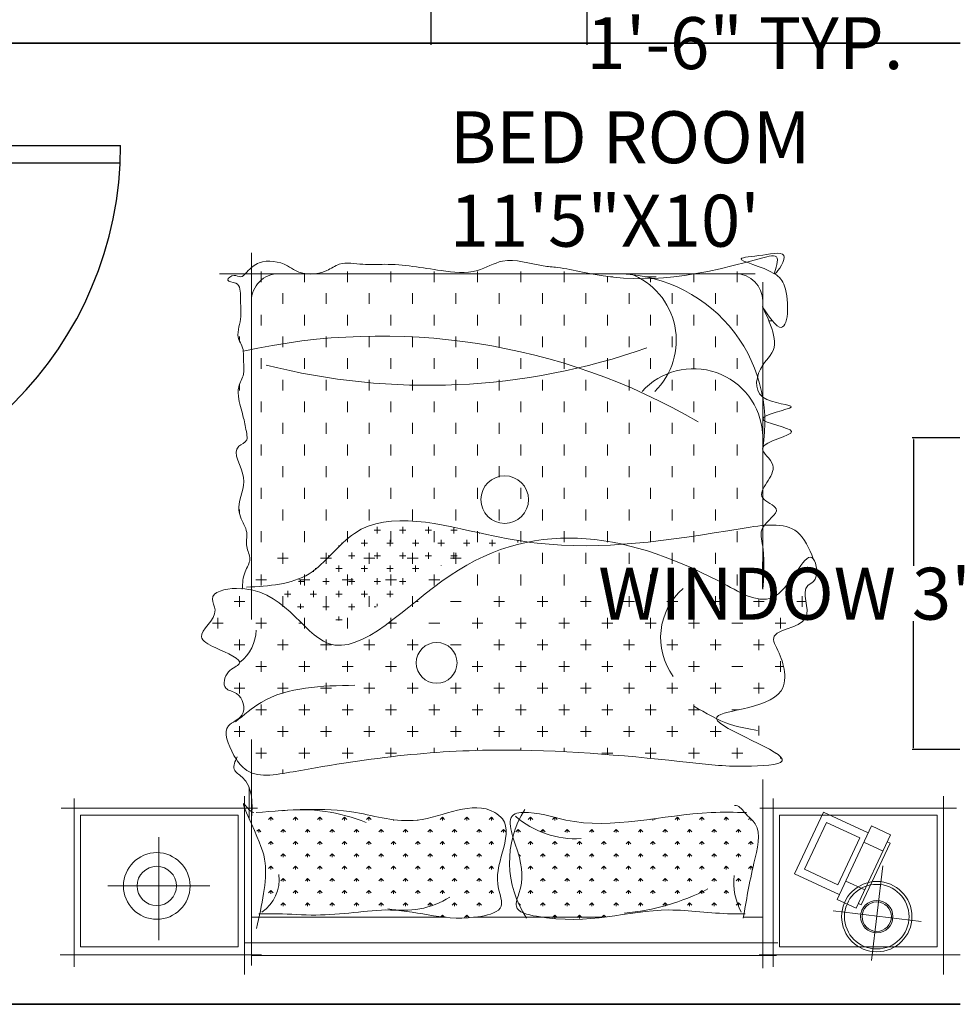
# Model space of a CAD drawing. Units: inches. Extents: x -26 to 575, y -18 to 513.
# Tile 17 of 28: x 405 to 513, y 128 to 241. Entities that reach past the tile are written whole.
import ezdxf

# ---------------------------------------------------------------- set-up
doc = ezdxf.new("R2010")
doc.units = ezdxf.units.IN
doc.header["$MEASUREMENT"] = 0
for name, color, linetype, lineweight in [('A-ANNO-DIMS', 2, 'Continuous', 18), ('A-AREA-IDEN', 7, 'Continuous', 18), ('A-DOOR', 3, 'Continuous', 25), ('A-WALL', 7, 'Continuous', 35), ('Furniture', 8, 'Continuous', 15)]:
    doc.layers.add(name, color=color, linetype=linetype, lineweight=lineweight)
doc.styles.get("Standard").update_dxf_attribs({"font": 'arial.ttf', "height": 6})
doc.dimstyles.get("Standard").update_dxf_attribs({"dimtxt": 6, "dimasz": 0.18, "dimexe": 0.18, "dimexo": 0.0625, "dimgap": 0.09, "dimtad": 0, "dimtih": 1, "dimtoh": 1, "dimzin": 0, "dimdsep": 46, "dimlunit": 3, "dimtxsty": 'Standard', "dimcen": 0.09, "dimadec": 0, "dimazin": 0, "dimtfac": 1, "dimtofl": 0, "dimtmove": 0, "dimatfit": 3, "dimfxl": 1, "dimtolj": 1, "dimtzin": 0, "dimarcsym": 0})

# ---------------------------------------------------------------- blocks, each defined once
blk = doc.blocks.new('BED-DOUBLE-WITH-NIGHTSTANDS')
for p, q in [((1.93, 83.36), (1.93, 62.76)), ((82.67, 83.36), (82.67, 62.76)), ((21.61, 63.03), (21.61, 82.46)), ((22.83, 60.83), (22.83, 82.62)), ((81.88, 82.34), (81.88, 56.23)), ((102.35, 63.03), (102.35, 82.46)), ((23.23, 81.08), (0, 81.08)), ((10.27, 81.76), (8.94, 70.83)), ((21.24, 81.17), (81.88, 81.17)), ((103.97, 81.08), (80.74, 81.08)), ((20.89, 80.15), (2.67, 80.15)), ((2.67, 80.15), (2.67, 64.97)), ((20.89, 64.97), (20.89, 80.15)), ((82.67, 79.72), (21.06, 79.72)), ((101.63, 80.15), (83.41, 80.15)), ((83.41, 80.15), (83.41, 64.97)), ((101.63, 64.97), (101.63, 80.15)), ((92.57, 79.4), (92.57, 67.51)), ((14.67, 76.01), (4.51, 77.26)), ((25.06, 76.76), (22.83, 76.76)), ((41.17, 76.51), (40.96, 76.72)), ((41.17, 76.51), (41.43, 76.77)), ((41.17, 76.51), (41.17, 76.74)), ((56.23, 76.76), (41.36, 76.76)), ((44, 76.51), (43.73, 76.77)), ((44, 76.51), (44, 76.88)), ((44, 76.51), (44.26, 76.77)), ((46.83, 76.51), (46.56, 76.77)), ((46.83, 76.51), (46.83, 76.88)), ((46.83, 76.51), (47.09, 76.77)), ((57, 76.51), (56.74, 76.77)), ((57, 76.51), (57, 76.83)), ((57, 76.51), (57.27, 76.77)), ((81.88, 76.76), (59.39, 76.76)), ((59.83, 76.51), (59.59, 76.74)), ((59.83, 76.51), (59.83, 76.72)), ((59.83, 76.51), (60.02, 76.69)), ((8.06, 67.24), (12.03, 75.72)), ((11.46, 75.32), (8.12, 68.2)), ((11.77, 75.18), (11.46, 75.32)), ((12.03, 75.72), (14.23, 74.69)), ((25.61, 75.09), (25.35, 75.36)), ((25.61, 75.09), (25.61, 75.47)), ((25.61, 75.09), (25.88, 75.36)), ((28.44, 75.09), (28.18, 75.36)), ((28.44, 75.09), (28.44, 75.47)), ((28.44, 75.09), (28.71, 75.36)), ((31.27, 75.09), (31, 75.36)), ((31.27, 75.09), (31.27, 75.47)), ((31.27, 75.09), (31.53, 75.36)), ((34.1, 75.09), (33.83, 75.36)), ((34.1, 75.09), (34.1, 75.47)), ((34.1, 75.09), (34.36, 75.36)), ((36.93, 75.09), (36.66, 75.36)), ((36.93, 75.09), (36.93, 75.47)), ((36.93, 75.09), (37.19, 75.36)), ((39.75, 75.09), (39.49, 75.36)), ((39.75, 75.09), (39.75, 75.47)), ((39.75, 75.09), (40.02, 75.36)), ((42.58, 75.09), (42.32, 75.36)), ((42.58, 75.09), (42.58, 75.47)), ((42.58, 75.09), (42.85, 75.36)), ((45.41, 75.09), (45.15, 75.36)), ((45.41, 75.09), (45.41, 75.47)), ((45.41, 75.09), (45.68, 75.36)), ((48.24, 75.09), (47.97, 75.36)), ((48.24, 75.09), (48.24, 75.47)), ((48.24, 75.09), (48.5, 75.36)), ((51.07, 75.09), (50.8, 75.36)), ((51.07, 75.09), (51.07, 75.1)), ((51.07, 75.09), (51.07, 75.1)), ((53, 75.34), (53.03, 75.36)), ((55.59, 75.09), (55.32, 75.36)), ((55.59, 75.09), (55.59, 75.47)), ((55.59, 75.09), (55.85, 75.36)), ((58.42, 75.09), (58.15, 75.36)), ((58.42, 75.09), (58.42, 75.47)), ((58.42, 75.09), (58.68, 75.36)), ((61.25, 75.09), (60.98, 75.36)), ((61.25, 75.09), (61.25, 75.47)), ((61.25, 75.09), (61.51, 75.36)), ((64.07, 75.09), (63.81, 75.36)), ((64.07, 75.09), (64.07, 75.47)), ((64.07, 75.09), (64.34, 75.36)), ((66.9, 75.09), (66.64, 75.36)), ((66.9, 75.09), (66.9, 75.47)), ((66.9, 75.09), (67.17, 75.36)), ((69.73, 75.09), (69.47, 75.36)), ((69.73, 75.09), (69.73, 75.47)), ((69.73, 75.09), (70, 75.36)), ((72.56, 75.09), (72.29, 75.36)), ((72.56, 75.09), (72.56, 75.47)), ((72.56, 75.09), (72.82, 75.36)), ((75.39, 75.09), (75.12, 75.36)), ((75.39, 75.09), (75.39, 75.47)), ((75.39, 75.09), (75.65, 75.36)), ((78.22, 75.09), (77.95, 75.36)), ((78.22, 75.09), (78.22, 75.47)), ((78.22, 75.09), (78.48, 75.36)), ((14.23, 74.69), (10.26, 66.21)), ((19.14, 71.73), (13.98, 74.14)), ((27.03, 73.68), (26.76, 73.94)), ((27.03, 73.68), (27.03, 74.05)), ((27.03, 73.68), (27.29, 73.94)), ((29.85, 73.68), (29.59, 73.94)), ((29.85, 73.68), (30.12, 73.94)), ((29.86, 73.68), (29.86, 74.05)), ((32.68, 73.68), (32.42, 73.94)), ((32.68, 73.68), (32.68, 74.05)), ((32.68, 73.68), (32.95, 73.94)), ((35.51, 73.68), (35.25, 73.94)), ((35.51, 73.68), (35.51, 74.05)), ((35.51, 73.68), (35.78, 73.94)), ((38.34, 73.68), (38.07, 73.94)), ((38.34, 73.68), (38.34, 74.05)), ((38.34, 73.68), (38.61, 73.94)), ((41.17, 73.68), (40.9, 73.94)), ((41.17, 73.68), (41.17, 74.05)), ((41.17, 73.68), (41.43, 73.94)), ((44, 73.68), (43.73, 73.94)), ((44, 73.68), (44, 74.05)), ((44, 73.68), (44.26, 73.94)), ((46.83, 73.68), (46.56, 73.94)), ((46.83, 73.68), (46.83, 74.05)), ((46.83, 73.68), (47.09, 73.94)), ((49.65, 73.68), (49.39, 73.94)), ((49.65, 73.68), (49.65, 74.05)), ((49.65, 73.68), (49.92, 73.94)), ((54.17, 73.68), (53.91, 73.94)), ((54.17, 73.68), (54.17, 74.05)), ((54.17, 73.68), (54.44, 73.94)), ((57, 73.68), (56.74, 73.94)), ((57, 73.68), (57, 74.05)), ((57, 73.68), (57.27, 73.94)), ((59.83, 73.68), (59.57, 73.94)), ((59.83, 73.68), (59.83, 74.05)), ((59.83, 73.68), (60.1, 73.94)), ((62.66, 73.68), (62.39, 73.94)), ((62.66, 73.68), (62.66, 74.05)), ((62.66, 73.68), (62.92, 73.94)), ((65.49, 73.68), (65.22, 73.94)), ((65.49, 73.68), (65.49, 74.05)), ((65.49, 73.68), (65.75, 73.94)), ((68.32, 73.68), (68.05, 73.94)), ((68.32, 73.68), (68.32, 74.05)), ((68.32, 73.68), (68.58, 73.94)), ((71.14, 73.68), (70.88, 73.94)), ((71.14, 73.68), (71.41, 73.94)), ((71.15, 73.68), (71.15, 74.05)), ((73.97, 73.68), (73.71, 73.94)), ((73.97, 73.68), (73.97, 74.05)), ((73.97, 73.68), (74.24, 73.94)), ((76.8, 73.68), (76.54, 73.94)), ((76.8, 73.68), (76.8, 74.05)), ((76.8, 73.68), (77.07, 73.94)), ((79.63, 73.68), (79.36, 73.94)), ((79.63, 73.68), (79.63, 74.05)), ((79.63, 73.68), (79.9, 73.94)), ((13.24, 72.57), (11.03, 73.6)), ((14.13, 73), (11.6, 67.59)), ((17.98, 71.2), (14.13, 73)), ((98.47, 73.14), (86.67, 73.14)), ((15.8, 64.6), (19.14, 71.73)), ((25.61, 72.26), (25.35, 72.53)), ((25.61, 72.26), (25.61, 72.64)), ((25.61, 72.26), (25.88, 72.53)), ((28.44, 72.26), (28.18, 72.53)), ((28.44, 72.26), (28.44, 72.64)), ((28.44, 72.26), (28.71, 72.53)), ((31.27, 72.26), (31, 72.53)), ((31.27, 72.26), (31.27, 72.64)), ((31.27, 72.26), (31.53, 72.53)), ((34.1, 72.26), (33.83, 72.53)), ((34.1, 72.26), (34.1, 72.64)), ((34.1, 72.26), (34.36, 72.53)), ((36.93, 72.26), (36.66, 72.53)), ((36.93, 72.26), (36.93, 72.64)), ((36.93, 72.26), (37.19, 72.53)), ((39.75, 72.26), (39.49, 72.53)), ((39.75, 72.26), (39.75, 72.64)), ((39.75, 72.26), (40.02, 72.53)), ((42.58, 72.26), (42.32, 72.53)), ((42.58, 72.26), (42.58, 72.64)), ((42.58, 72.26), (42.85, 72.53)), ((45.41, 72.26), (45.15, 72.53)), ((45.41, 72.26), (45.41, 72.64)), ((45.41, 72.26), (45.68, 72.53)), ((48.24, 72.26), (47.97, 72.53)), ((48.24, 72.26), (48.24, 72.64)), ((48.24, 72.26), (48.5, 72.53)), ((55.59, 72.26), (55.32, 72.53)), ((55.59, 72.26), (55.59, 72.64)), ((55.59, 72.26), (55.85, 72.53)), ((58.42, 72.26), (58.15, 72.53)), ((58.42, 72.26), (58.42, 72.64)), ((58.42, 72.26), (58.68, 72.53)), ((61.25, 72.26), (60.98, 72.53)), ((61.25, 72.26), (61.25, 72.64)), ((61.25, 72.26), (61.51, 72.53)), ((64.07, 72.26), (63.81, 72.53)), ((64.07, 72.26), (64.07, 72.64)), ((64.07, 72.26), (64.34, 72.53)), ((66.9, 72.26), (66.64, 72.53)), ((66.9, 72.26), (66.9, 72.64)), ((66.9, 72.26), (67.17, 72.53)), ((69.73, 72.26), (69.47, 72.53)), ((69.73, 72.26), (69.73, 72.64)), ((69.73, 72.26), (70, 72.53)), ((72.56, 72.26), (72.29, 72.53)), ((72.56, 72.26), (72.56, 72.64)), ((72.56, 72.26), (72.82, 72.53)), ((75.39, 72.26), (75.12, 72.53)), ((75.39, 72.26), (75.39, 72.64)), ((75.39, 72.26), (75.65, 72.53)), ((78.22, 72.26), (77.95, 72.53)), ((78.22, 72.26), (78.22, 72.64)), ((78.22, 72.26), (78.48, 72.53)), ((15.45, 65.79), (17.98, 71.2)), ((24.2, 70.85), (23.97, 71.08)), ((24.2, 70.85), (24.2, 71.23)), ((24.2, 70.85), (24.46, 71.12)), ((27.03, 70.85), (26.76, 71.12)), ((27.03, 70.85), (27.03, 71.23)), ((27.03, 70.85), (27.29, 71.12)), ((29.85, 70.85), (29.59, 71.12)), ((29.85, 70.85), (30.12, 71.12)), ((29.86, 70.85), (29.86, 71.23)), ((32.68, 70.85), (32.42, 71.12)), ((32.68, 70.85), (32.68, 71.23)), ((32.68, 70.85), (32.95, 71.12)), ((35.51, 70.85), (35.25, 71.12)), ((35.51, 70.85), (35.51, 71.23)), ((35.51, 70.85), (35.78, 71.12)), ((38.34, 70.85), (38.07, 71.12)), ((38.34, 70.85), (38.34, 71.23)), ((38.34, 70.85), (38.61, 71.12)), ((41.17, 70.85), (40.9, 71.12)), ((41.17, 70.85), (41.17, 71.23)), ((41.17, 70.85), (41.43, 71.12)), ((44, 70.85), (43.73, 71.12)), ((44, 70.85), (44, 71.23)), ((44, 70.85), (44.26, 71.12)), ((46.83, 70.85), (46.56, 71.12)), ((46.83, 70.85), (46.83, 71.23)), ((46.83, 70.85), (47.09, 71.12)), ((49.65, 70.85), (49.39, 71.12)), ((49.65, 70.85), (49.65, 71.23)), ((49.65, 70.85), (49.92, 71.12)), ((54.17, 70.85), (53.91, 71.12)), ((54.17, 70.85), (54.17, 71.23)), ((54.17, 70.85), (54.44, 71.12)), ((57, 70.85), (56.74, 71.12)), ((57, 70.85), (57, 71.23)), ((57, 70.85), (57.27, 71.12)), ((59.83, 70.85), (59.57, 71.12)), ((59.83, 70.85), (59.83, 71.23)), ((59.83, 70.85), (60.1, 71.12)), ((62.66, 70.85), (62.39, 71.12)), ((62.66, 70.85), (62.66, 71.23)), ((62.66, 70.85), (62.92, 71.12)), ((65.49, 70.85), (65.22, 71.12)), ((65.49, 70.85), (65.49, 71.23)), ((65.49, 70.85), (65.75, 71.12)), ((68.32, 70.85), (68.05, 71.12)), ((68.32, 70.85), (68.32, 71.23)), ((68.32, 70.85), (68.58, 71.12)), ((71.14, 70.85), (70.88, 71.12)), ((71.14, 70.85), (71.41, 71.12)), ((71.15, 70.85), (71.15, 71.23)), ((73.97, 70.85), (73.71, 71.12)), ((73.97, 70.85), (73.97, 71.23)), ((73.97, 70.85), (74.24, 71.12)), ((76.8, 70.85), (76.54, 71.12)), ((76.8, 70.85), (76.8, 71.23)), ((76.8, 70.85), (77.07, 71.12)), ((79.63, 70.85), (79.36, 71.12)), ((79.63, 70.85), (79.63, 71.23)), ((79.63, 70.85), (79.9, 71.12)), ((25.61, 69.44), (25.35, 69.7)), ((25.61, 69.44), (25.61, 69.81)), ((25.61, 69.44), (25.88, 69.7)), ((28.44, 69.44), (28.18, 69.7)), ((28.44, 69.44), (28.44, 69.81)), ((28.44, 69.44), (28.71, 69.7)), ((31.27, 69.44), (31, 69.7)), ((31.27, 69.44), (31.27, 69.81)), ((31.27, 69.44), (31.53, 69.7)), ((34.1, 69.44), (33.83, 69.7)), ((34.1, 69.44), (34.1, 69.81)), ((34.1, 69.44), (34.36, 69.7)), ((36.93, 69.44), (36.66, 69.7)), ((36.93, 69.44), (36.93, 69.81)), ((36.93, 69.44), (37.19, 69.7)), ((39.75, 69.44), (39.49, 69.7)), ((39.75, 69.44), (39.75, 69.81)), ((39.75, 69.44), (40.02, 69.7)), ((42.58, 69.44), (42.32, 69.7)), ((42.58, 69.44), (42.58, 69.81)), ((42.58, 69.44), (42.85, 69.7)), ((45.41, 69.44), (45.15, 69.7)), ((45.41, 69.44), (45.41, 69.81)), ((45.41, 69.44), (45.68, 69.7)), ((48.24, 69.44), (47.97, 69.7)), ((48.24, 69.44), (48.24, 69.81)), ((48.24, 69.44), (48.5, 69.7)), ((51.05, 69.45), (50.8, 69.7)), ((53.01, 69.68), (53.03, 69.7)), ((55.59, 69.44), (55.32, 69.7)), ((55.59, 69.44), (55.59, 69.81)), ((55.59, 69.44), (55.85, 69.7)), ((58.42, 69.44), (58.15, 69.7)), ((58.42, 69.44), (58.42, 69.81)), ((58.42, 69.44), (58.68, 69.7)), ((61.25, 69.44), (60.98, 69.7)), ((61.25, 69.44), (61.25, 69.81)), ((61.25, 69.44), (61.51, 69.7)), ((64.07, 69.44), (63.81, 69.7)), ((64.07, 69.44), (64.07, 69.81)), ((64.07, 69.44), (64.34, 69.7)), ((66.9, 69.44), (66.64, 69.7)), ((66.9, 69.44), (66.9, 69.81)), ((66.9, 69.44), (67.17, 69.7)), ((69.73, 69.44), (69.47, 69.7)), ((69.73, 69.44), (69.73, 69.81)), ((69.73, 69.44), (70, 69.7)), ((72.56, 69.44), (72.29, 69.7)), ((72.56, 69.44), (72.56, 69.81)), ((72.56, 69.44), (72.82, 69.7)), ((75.39, 69.44), (75.12, 69.7)), ((75.39, 69.44), (75.39, 69.81)), ((75.39, 69.44), (75.65, 69.7)), ((78.22, 69.44), (77.95, 69.7)), ((78.22, 69.44), (78.22, 69.81)), ((78.22, 69.44), (78.48, 69.7)), ((11.14, 68.07), (8.93, 69.1)), ((24.2, 68.02), (23.93, 68.29)), ((24.2, 68.02), (24.2, 68.4)), ((24.2, 68.02), (24.46, 68.29)), ((27.03, 68.02), (26.76, 68.29)), ((27.03, 68.02), (27.03, 68.4)), ((27.03, 68.02), (27.29, 68.29)), ((29.85, 68.02), (29.59, 68.29)), ((29.85, 68.02), (30.12, 68.29)), ((29.86, 68.02), (29.86, 68.4)), ((32.68, 68.02), (32.42, 68.29)), ((32.68, 68.02), (32.68, 68.4)), ((32.68, 68.02), (32.95, 68.29)), ((35.51, 68.02), (35.25, 68.29)), ((35.51, 68.02), (35.51, 68.4)), ((35.51, 68.02), (35.78, 68.29)), ((38.34, 68.02), (38.07, 68.29)), ((38.34, 68.02), (38.34, 68.4)), ((38.34, 68.02), (38.61, 68.29)), ((41.17, 68.02), (40.9, 68.29)), ((41.17, 68.02), (41.17, 68.4)), ((41.17, 68.02), (41.43, 68.29)), ((44, 68.02), (43.73, 68.29)), ((44, 68.02), (44, 68.4)), ((44, 68.02), (44.26, 68.29)), ((46.83, 68.02), (46.56, 68.29)), ((46.83, 68.02), (46.83, 68.4)), ((46.83, 68.02), (47.09, 68.29)), ((49.65, 68.02), (49.39, 68.29)), ((49.65, 68.02), (49.65, 68.4)), ((49.65, 68.02), (49.92, 68.29)), ((54.17, 68.02), (53.91, 68.29)), ((54.17, 68.02), (54.17, 68.4)), ((54.17, 68.02), (54.44, 68.29)), ((57, 68.02), (56.74, 68.29)), ((57, 68.02), (57, 68.4)), ((57, 68.02), (57.27, 68.29)), ((59.83, 68.02), (59.57, 68.29)), ((59.83, 68.02), (59.83, 68.4)), ((59.83, 68.02), (60.1, 68.29)), ((62.66, 68.02), (62.39, 68.29)), ((62.66, 68.02), (62.66, 68.4)), ((62.66, 68.02), (62.92, 68.29)), ((65.49, 68.02), (65.22, 68.29)), ((65.49, 68.02), (65.49, 68.4)), ((65.49, 68.02), (65.75, 68.29)), ((68.32, 68.02), (68.05, 68.29)), ((68.32, 68.02), (68.32, 68.4)), ((68.32, 68.02), (68.58, 68.29)), ((71.14, 68.02), (70.88, 68.29)), ((71.14, 68.02), (71.41, 68.29)), ((71.15, 68.02), (71.15, 68.4)), ((73.97, 68.02), (73.71, 68.29)), ((73.97, 68.02), (73.97, 68.4)), ((73.97, 68.02), (74.24, 68.29)), ((76.8, 68.02), (76.54, 68.29)), ((76.8, 68.02), (76.8, 68.4)), ((76.8, 68.02), (77.07, 68.29)), ((79.63, 68.02), (79.36, 68.29)), ((79.63, 68.02), (79.63, 68.4)), ((79.63, 68.02), (79.9, 68.29)), ((10.26, 66.21), (8.06, 67.24)), ((8.12, 68.2), (8.43, 68.05)), ((11.6, 67.59), (15.45, 65.79)), ((10.64, 67.02), (15.8, 64.6)), ((25.61, 66.61), (25.35, 66.87)), ((25.61, 66.61), (25.61, 66.98)), ((25.61, 66.61), (25.88, 66.87)), ((28.44, 66.61), (28.18, 66.87)), ((28.44, 66.61), (28.44, 66.98)), ((28.44, 66.61), (28.71, 66.87)), ((31.27, 66.61), (31, 66.87)), ((31.27, 66.61), (31.27, 66.98)), ((31.27, 66.61), (31.53, 66.87)), ((34.1, 66.61), (33.83, 66.87)), ((34.1, 66.61), (34.1, 66.98)), ((34.1, 66.61), (34.36, 66.87)), ((36.93, 66.61), (36.66, 66.87)), ((36.93, 66.61), (36.93, 66.98)), ((36.93, 66.61), (37.19, 66.87)), ((39.75, 66.61), (39.49, 66.87)), ((39.75, 66.61), (39.75, 66.98)), ((39.75, 66.61), (40.02, 66.87)), ((42.58, 66.61), (42.32, 66.87)), ((42.58, 66.61), (42.58, 66.98)), ((42.58, 66.61), (42.85, 66.87)), ((45.41, 66.61), (45.15, 66.87)), ((45.41, 66.61), (45.41, 66.98)), ((45.41, 66.61), (45.68, 66.87)), ((48.24, 66.61), (47.97, 66.87)), ((48.24, 66.61), (48.24, 66.98)), ((48.24, 66.61), (48.5, 66.87)), ((51.07, 66.61), (50.8, 66.87)), ((51.07, 66.61), (51.07, 66.98)), ((51.07, 66.61), (51.33, 66.87)), ((52.76, 66.61), (52.49, 66.87)), ((52.76, 66.61), (52.76, 66.98)), ((52.76, 66.61), (53.03, 66.87)), ((55.59, 66.61), (55.32, 66.87)), ((55.59, 66.61), (55.59, 66.98)), ((55.59, 66.61), (55.85, 66.87)), ((58.42, 66.61), (58.15, 66.87)), ((58.42, 66.61), (58.42, 66.98)), ((58.42, 66.61), (58.68, 66.87)), ((61.25, 66.61), (60.98, 66.87)), ((61.25, 66.61), (61.25, 66.98)), ((61.25, 66.61), (61.51, 66.87)), ((64.07, 66.61), (63.81, 66.87)), ((64.07, 66.61), (64.07, 66.98)), ((64.07, 66.61), (64.34, 66.87)), ((66.9, 66.61), (66.64, 66.87)), ((66.9, 66.61), (66.9, 66.98)), ((66.9, 66.61), (67.17, 66.87)), ((69.73, 66.61), (69.47, 66.87)), ((69.73, 66.61), (69.73, 66.98)), ((69.73, 66.61), (70, 66.87)), ((72.56, 66.61), (72.29, 66.87)), ((72.56, 66.61), (72.56, 66.98)), ((72.56, 66.61), (72.82, 66.87)), ((75.39, 66.61), (75.12, 66.87)), ((75.39, 66.61), (75.39, 66.98)), ((75.39, 66.61), (75.65, 66.87)), ((78.22, 66.61), (77.95, 66.87)), ((78.22, 66.61), (78.22, 66.98)), ((78.22, 66.61), (78.48, 66.87)), ((81.04, 66.61), (80.78, 66.87)), ((81.04, 66.61), (81.04, 66.98)), ((81.04, 66.61), (81.25, 66.82)), ((2.67, 64.97), (20.89, 64.97)), ((24.2, 65.39), (24.2, 65.57)), ((24.29, 65.29), (24.46, 65.46)), ((27.03, 65.19), (26.76, 65.46)), ((27.03, 65.19), (27.03, 65.57)), ((27.03, 65.19), (27.29, 65.46)), ((29.85, 65.19), (29.59, 65.46)), ((29.85, 65.19), (30.12, 65.46)), ((29.86, 65.19), (29.86, 65.57)), ((32.68, 65.19), (32.42, 65.46)), ((32.68, 65.19), (32.68, 65.57)), ((32.68, 65.19), (32.95, 65.46)), ((35.33, 65.37), (35.25, 65.46)), ((35.51, 65.39), (35.51, 65.57)), ((35.74, 65.42), (35.78, 65.46)), ((46.77, 65.25), (46.56, 65.46)), ((46.83, 65.23), (46.83, 65.57)), ((46.86, 65.22), (47.09, 65.46)), ((49.65, 65.19), (49.39, 65.46)), ((49.65, 65.19), (49.65, 65.57)), ((49.65, 65.19), (49.92, 65.46)), ((54.17, 65.19), (53.91, 65.46)), ((54.17, 65.19), (54.17, 65.57)), ((54.17, 65.19), (54.44, 65.46)), ((57, 65.19), (56.74, 65.46)), ((57, 65.19), (57, 65.57)), ((57, 65.19), (57.27, 65.46)), ((59.83, 65.19), (59.57, 65.46)), ((59.83, 65.19), (59.83, 65.57)), ((59.83, 65.19), (60.1, 65.46)), ((62.66, 65.52), (62.66, 65.57)), ((65.49, 65.48), (65.49, 65.57)), ((65.74, 65.45), (65.75, 65.46)), ((68.32, 65.19), (68.05, 65.46)), ((68.32, 65.19), (68.32, 65.57)), ((68.32, 65.19), (68.58, 65.46)), ((71.14, 65.19), (70.88, 65.46)), ((71.14, 65.19), (71.41, 65.46)), ((71.15, 65.19), (71.15, 65.57)), ((73.97, 65.19), (73.71, 65.46)), ((73.97, 65.19), (73.97, 65.57)), ((73.97, 65.19), (74.24, 65.46)), ((76.8, 65.19), (76.54, 65.46)), ((76.8, 65.19), (76.8, 65.57)), ((76.8, 65.19), (77.07, 65.46)), ((79.63, 65.19), (79.36, 65.46)), ((79.63, 65.19), (79.63, 65.57)), ((79.63, 65.19), (79.9, 65.46)), ((82.15, 61.74), (82.15, 65.42)), ((83.41, 64.97), (101.63, 64.97)), ((0.45, 64.15), (23.14, 64.15)), ((55.59, 64.12), (55.59, 64.15)), ((81.19, 64.15), (103.88, 64.15)), ((78.27, 59.67), (78.27, 60.15)), ((20.77, 58.21), (20.77, 58.42)), ((25.77, 57.17), (25.77, 58.42)), ((30.77, 57.17), (30.77, 58.42)), ((35.77, 57.17), (35.77, 58.41)), ((65.77, 57.17), (65.77, 58.21)), ((70.77, 57.17), (70.77, 58.42)), ((75.77, 57.17), (75.77, 58.42)), ((80.77, 57.17), (80.77, 58.42)), ((21.39, 57.79), (21.31, 57.79)), ((26.39, 57.79), (25.14, 57.79)), ((31.39, 57.79), (30.14, 57.79)), ((36.39, 57.79), (35.14, 57.79)), ((41.39, 57.79), (40.14, 57.79)), ((40.77, 57.17), (40.77, 57.97)), ((45.77, 57.17), (45.77, 57.64)), ((50.77, 57.17), (50.77, 57.46)), ((55.77, 57.17), (55.77, 57.48)), ((60.77, 57.17), (60.77, 57.74)), ((66.39, 57.79), (65.14, 57.79)), ((71.39, 57.79), (70.14, 57.79)), ((76.39, 57.79), (75.14, 57.79)), ((81.39, 57.79), (80.14, 57.79)), ((23.27, 54.64), (23.27, 55.76)), ((28.27, 54.67), (28.27, 55.92)), ((33.27, 54.67), (33.27, 55.92)), ((38.27, 54.67), (38.27, 55.92)), ((43.27, 54.67), (43.27, 55.92)), ((48.27, 54.67), (48.27, 55.92)), ((53.27, 54.67), (53.27, 55.92)), ((58.27, 54.67), (58.27, 55.92)), ((63.27, 54.67), (63.27, 55.92)), ((68.27, 54.67), (68.27, 55.92)), ((73.27, 54.67), (73.27, 55.92)), ((78.27, 54.67), (78.27, 55.92)), ((83.27, 54.67), (83.27, 55.92)), ((28.89, 55.29), (27.64, 55.29)), ((33.89, 55.29), (32.64, 55.29)), ((38.89, 55.29), (37.64, 55.29)), ((43.89, 55.29), (42.64, 55.29)), ((48.89, 55.29), (47.64, 55.29)), ((53.89, 55.29), (52.64, 55.29)), ((58.89, 55.29), (57.64, 55.29)), ((63.89, 55.29), (62.64, 55.29)), ((68.89, 55.29), (67.64, 55.29)), ((73.89, 55.29), (72.64, 55.29)), ((78.89, 55.29), (77.64, 55.29)), ((83.89, 55.29), (82.64, 55.29)), ((26.39, 52.79), (25.62, 52.79)), ((31.39, 52.79), (30.14, 52.79)), ((30.77, 52.17), (30.77, 53.42)), ((36.39, 52.79), (35.14, 52.79)), ((35.77, 52.17), (35.77, 53.42)), ((41.39, 52.79), (40.14, 52.79)), ((40.77, 52.17), (40.77, 53.42)), ((46.39, 52.79), (45.14, 52.79)), ((45.77, 52.17), (45.77, 53.42)), ((51.39, 52.79), (50.14, 52.79)), ((50.77, 52.17), (50.77, 53.42)), ((56.39, 52.79), (55.14, 52.79)), ((55.77, 52.17), (55.77, 53.42)), ((61.39, 52.79), (60.14, 52.79)), ((60.77, 52.17), (60.77, 53.42)), ((66.39, 52.79), (65.14, 52.79)), ((65.77, 52.17), (65.77, 53.42)), ((71.39, 52.79), (70.14, 52.79)), ((70.77, 52.17), (70.77, 53.42)), ((76.39, 52.79), (75.14, 52.79)), ((75.77, 52.17), (75.77, 53.42)), ((81.39, 52.79), (80.14, 52.79)), ((80.77, 52.17), (80.77, 53.42)), ((23.89, 50.29), (22.64, 50.29)), ((23.27, 49.67), (23.27, 50.92)), ((28.89, 50.29), (27.64, 50.29)), ((28.27, 49.67), (28.27, 50.92)), ((33.89, 50.29), (32.64, 50.29)), ((33.27, 49.67), (33.27, 50.92)), ((38.89, 50.29), (37.64, 50.29)), ((38.27, 49.67), (38.27, 50.92)), ((43.89, 50.29), (42.64, 50.29)), ((43.27, 49.67), (43.27, 50.92)), ((48.89, 50.29), (47.64, 50.29)), ((48.27, 49.67), (48.27, 50.92)), ((53.89, 50.29), (52.64, 50.29)), ((53.27, 49.67), (53.27, 50.92)), ((58.89, 50.29), (57.64, 50.29)), ((58.27, 49.67), (58.27, 50.92)), ((63.89, 50.29), (62.64, 50.29)), ((63.27, 49.67), (63.27, 50.92)), ((68.89, 50.29), (67.64, 50.29)), ((68.27, 49.67), (68.27, 50.92)), ((73.89, 50.29), (72.64, 50.29)), ((73.27, 49.67), (73.27, 50.92)), ((78.89, 50.29), (77.64, 50.29)), ((78.27, 49.67), (78.27, 50.92)), ((83.89, 50.29), (82.64, 50.29)), ((83.27, 49.67), (83.27, 50.92)), ((21.39, 47.79), (20.41, 47.79)), ((20.77, 47.17), (20.77, 48.42)), ((26.39, 47.79), (25.14, 47.79)), ((31.39, 47.79), (30.14, 47.79)), ((30.77, 47.17), (30.77, 48.42)), ((36.39, 47.79), (35.14, 47.79)), ((35.77, 47.17), (35.77, 48.42)), ((41.39, 47.79), (40.14, 47.79)), ((40.77, 47.17), (40.77, 48.42)), ((46.39, 47.79), (45.14, 47.79)), ((45.77, 47.17), (45.77, 48.42)), ((51.39, 47.79), (50.14, 47.79)), ((50.77, 47.17), (50.77, 48.42)), ((56.39, 47.79), (55.14, 47.79)), ((55.77, 47.17), (55.77, 48.42)), ((66.39, 47.79), (65.14, 47.79)), ((65.77, 47.17), (65.77, 48.42)), ((71.39, 47.79), (70.14, 47.79)), ((70.77, 47.17), (70.77, 48.42)), ((76.39, 47.79), (75.14, 47.79)), ((75.77, 47.17), (75.77, 48.42)), ((81.39, 47.79), (80.14, 47.79)), ((80.77, 47.17), (80.77, 48.42)), ((23.27, 44.67), (23.27, 45.92)), ((28.27, 44.67), (28.27, 45.92)), ((33.27, 44.67), (33.27, 45.92)), ((38.27, 44.67), (38.27, 45.92)), ((43.27, 44.67), (43.27, 45.92)), ((48.27, 44.67), (48.27, 45.92)), ((53.27, 44.67), (53.27, 45.92)), ((63.27, 44.67), (63.27, 45.92)), ((68.27, 44.67), (68.27, 45.92)), ((73.27, 44.67), (73.27, 45.92)), ((78.27, 44.67), (78.27, 45.92)), ((83.27, 44.67), (83.27, 45.92)), ((23.89, 45.29), (22.64, 45.29)), ((28.89, 45.29), (27.64, 45.29)), ((33.89, 45.29), (32.64, 45.29)), ((38.89, 45.29), (37.64, 45.29)), ((43.89, 45.29), (42.64, 45.29)), ((48.89, 45.29), (47.64, 45.29)), ((53.89, 45.29), (52.64, 45.29)), ((58.89, 45.29), (57.64, 45.29)), ((63.89, 45.29), (62.64, 45.29)), ((68.89, 45.29), (67.64, 45.29)), ((73.89, 45.29), (72.64, 45.29)), ((78.89, 45.29), (77.64, 45.29)), ((83.89, 45.29), (82.64, 45.29)), ((20.77, 42.17), (20.77, 43.42)), ((30.77, 42.17), (30.77, 43.42)), ((35.77, 42.17), (35.77, 43.42)), ((40.77, 42.17), (40.77, 43.42)), ((45.77, 42.17), (45.77, 43.42)), ((50.77, 42.17), (50.77, 43.42)), ((55.77, 42.17), (55.77, 43.42)), ((65.77, 42.17), (65.77, 43.42)), ((70.77, 42.17), (70.77, 43.42)), ((75.77, 42.17), (75.77, 43.42)), ((80.77, 42.17), (80.77, 43.42)), ((85.77, 42.17), (85.77, 43.42)), ((21.39, 42.79), (20.14, 42.79)), ((26.39, 42.79), (25.14, 42.79)), ((31.39, 42.79), (30.14, 42.79)), ((36.39, 42.79), (35.14, 42.79)), ((41.39, 42.79), (40.14, 42.79)), ((46.39, 42.79), (45.14, 42.79)), ((51.39, 42.79), (50.14, 42.79)), ((56.39, 42.79), (55.14, 42.79)), ((61.39, 42.79), (60.14, 42.79)), ((66.09, 42.79), (65.14, 42.79)), ((72.15, 42.39), (71.41, 42.39)), ((71.78, 42.02), (71.78, 42.49)), ((76.39, 42.79), (76.07, 42.79)), ((81.39, 42.79), (80.14, 42.79)), ((81.88, 42.36), (81.88, 0)), ((86.39, 42.79), (85.14, 42.79)), ((70.3, 40.54), (70.3, 41.28)), ((73.26, 40.54), (73.26, 41.28)), ((76.21, 40.54), (76.21, 41.13)), ((18.89, 40.29), (17.83, 40.29)), ((18.27, 39.67), (18.27, 40.92)), ((23.89, 40.29), (22.64, 40.29)), ((23.27, 39.99), (23.27, 40.92)), ((28.89, 40.29), (27.64, 40.29)), ((28.27, 39.67), (28.27, 40.92)), ((33.89, 40.29), (32.64, 40.29)), ((33.27, 39.67), (33.27, 40.92)), ((38.89, 40.29), (37.64, 40.29)), ((38.27, 39.67), (38.27, 40.92)), ((43.89, 40.29), (42.64, 40.29)), ((43.27, 39.67), (43.27, 40.92)), ((48.89, 40.29), (47.64, 40.29)), ((48.27, 39.67), (48.27, 40.92)), ((53.89, 40.29), (52.64, 40.29)), ((53.27, 39.67), (53.27, 40.92)), ((58.89, 40.29), (57.64, 40.29)), ((62.9, 40.29), (62.64, 40.29)), ((63.27, 39.67), (63.27, 40.92)), ((65.87, 39.06), (65.87, 39.8)), ((67.35, 40.54), (67.35, 40.84)), ((67.72, 40.91), (67.48, 40.91)), ((68.27, 39.67), (68.27, 40.92)), ((68.83, 39.06), (68.83, 39.8)), ((70.67, 40.91), (69.93, 40.91)), ((71.78, 39.06), (71.78, 39.8)), ((73.62, 40.91), (72.89, 40.91)), ((73.27, 39.67), (73.27, 40.92)), ((74.73, 39.06), (74.73, 39.8)), ((76.58, 40.91), (75.84, 40.91)), ((77.68, 39.06), (77.68, 39.8)), ((78.27, 39.67), (78.27, 40.92)), ((83.89, 40.29), (82.64, 40.29)), ((83.27, 39.67), (83.27, 40.92)), ((22.83, 3.42), (22.83, 38.86)), ((66.24, 39.43), (65.5, 39.43)), ((69.2, 39.43), (68.46, 39.43)), ((72.15, 39.43), (71.41, 39.43)), ((75.1, 39.43), (74.36, 39.43)), ((78.05, 39.43), (77.32, 39.43)), ((25.77, 37.17), (25.77, 38.42)), ((30.77, 37.17), (30.77, 38.42)), ((35.77, 37.17), (35.77, 38.42)), ((40.77, 37.17), (40.77, 38.42)), ((45.77, 37.17), (45.77, 38.42)), ((50.77, 37.17), (50.77, 38.42)), ((55.77, 37.17), (55.77, 38.42)), ((61.39, 37.79), (60.14, 37.79)), ((60.77, 37.17), (60.77, 38.42)), ((64.77, 37.96), (64.03, 37.96)), ((64.4, 37.59), (64.4, 38.33)), ((66.39, 37.79), (65.14, 37.79)), ((65.77, 37.17), (65.77, 38.42)), ((67.72, 37.96), (66.98, 37.96)), ((67.35, 37.59), (67.35, 38.33)), ((70.67, 37.96), (69.93, 37.96)), ((71.39, 37.79), (70.14, 37.79)), ((70.3, 37.59), (70.3, 38.33)), ((70.77, 37.17), (70.77, 38.42)), ((73.62, 37.96), (72.89, 37.96)), ((73.26, 37.59), (73.26, 38.33)), ((76.39, 37.79), (75.14, 37.79)), ((75.77, 37.17), (75.77, 38.42)), ((76.45, 37.96), (75.84, 37.96)), ((76.21, 37.8), (76.21, 38.33)), ((81.39, 37.79), (80.14, 37.79)), ((80.77, 37.17), (80.77, 38.42)), ((63.29, 36.48), (62.55, 36.48)), ((62.92, 36.11), (62.92, 36.85)), ((66.24, 36.48), (65.5, 36.48)), ((65.87, 36.11), (65.87, 36.85)), ((69.2, 36.48), (68.46, 36.48)), ((68.83, 36.11), (68.83, 36.85)), ((72.15, 36.48), (71.41, 36.48)), ((71.78, 36.11), (71.78, 36.85)), ((74.53, 36.48), (74.36, 36.48)), ((74.73, 36.66), (74.73, 36.85)), ((17.66, 35.29), (17.64, 35.29)), ((28.27, 34.67), (28.27, 35.92)), ((33.27, 34.67), (33.27, 35.92)), ((38.27, 34.67), (38.27, 35.92)), ((43.27, 34.67), (43.27, 35.92)), ((48.27, 34.67), (48.27, 35.92)), ((53.27, 34.67), (53.27, 35.92)), ((58.89, 35.29), (57.64, 35.29)), ((58.27, 34.67), (58.27, 35.92)), ((58.49, 34.64), (58.49, 35.37)), ((59.97, 36.11), (59.97, 36.16)), ((61.44, 34.64), (61.44, 35.37)), ((63.89, 35.29), (62.64, 35.29)), ((63.27, 34.67), (63.27, 35.92)), ((64.4, 34.64), (64.4, 35.37)), ((67.35, 34.64), (67.35, 35.37)), ((68.89, 35.29), (67.64, 35.29)), ((68.27, 34.67), (68.27, 35.92)), ((70.3, 34.64), (70.3, 35.37)), ((73.89, 35.29), (72.64, 35.29)), ((73.26, 35.25), (73.26, 35.37)), ((73.27, 34.67), (73.27, 35.92)), ((78.89, 35.29), (77.64, 35.29)), ((78.27, 34.67), (78.27, 35.92)), ((58.86, 35), (58.12, 35)), ((61.81, 35), (61.08, 35)), ((64.77, 35), (64.03, 35)), ((67.72, 35), (66.98, 35)), ((70.67, 35), (69.93, 35)), ((73.01, 35), (72.89, 35)), ((25.77, 32.17), (25.77, 33.42)), ((30.77, 32.17), (30.77, 33.42)), ((35.77, 32.17), (35.77, 33.42)), ((40.77, 32.17), (40.77, 33.42)), ((45.77, 32.17), (45.77, 33.42)), ((50.77, 32.17), (50.77, 33.42)), ((51.11, 33.25), (51.11, 33.48)), ((54.43, 33.53), (53.69, 33.53)), ((54.06, 33.16), (54.06, 33.9)), ((55.77, 32.17), (55.77, 33.42)), ((57.38, 33.53), (56.65, 33.53)), ((57.02, 33.16), (57.02, 33.9)), ((60.34, 33.53), (59.6, 33.53)), ((59.97, 33.16), (59.97, 33.9)), ((60.77, 32.17), (60.77, 33.42)), ((63.29, 33.53), (62.55, 33.53)), ((62.92, 33.16), (62.92, 33.9)), ((66.24, 33.53), (65.5, 33.53)), ((65.77, 32.17), (65.77, 33.42)), ((65.87, 33.16), (65.87, 33.9)), ((69.2, 33.53), (68.46, 33.53)), ((68.83, 33.16), (68.83, 33.9)), ((70.77, 32.17), (70.77, 33.42)), ((71.47, 33.53), (71.41, 33.53)), ((71.78, 33.81), (71.78, 33.9)), ((75.77, 32.17), (75.77, 33.42)), ((80.77, 32.17), (80.77, 33.42)), ((55.54, 32.37), (55.54, 32.42)), ((58.86, 32.05), (58.12, 32.05)), ((58.49, 31.74), (58.49, 32.42)), ((61.81, 32.05), (61.08, 32.05)), ((61.44, 31.68), (61.44, 32.42)), ((64.77, 32.05), (64.03, 32.05)), ((64.4, 31.68), (64.4, 32.42)), ((67.72, 32.05), (66.98, 32.05)), ((67.35, 31.68), (67.35, 32.42)), ((28.27, 29.67), (28.27, 30.92)), ((33.27, 29.67), (33.27, 30.92)), ((38.27, 29.67), (38.27, 30.92)), ((43.27, 29.67), (43.27, 30.92)), ((48.27, 29.67), (48.27, 30.92)), ((53.27, 29.67), (53.27, 30.92)), ((58.27, 29.67), (58.27, 30.92)), ((63.27, 29.67), (63.27, 30.92)), ((68.27, 29.67), (68.27, 30.92)), ((73.27, 29.67), (73.27, 30.92)), ((78.27, 29.67), (78.27, 30.92)), ((83.27, 29.67), (83.27, 30.11)), ((25.77, 27.17), (25.77, 28.42)), ((30.77, 27.17), (30.77, 28.42)), ((35.77, 27.17), (35.77, 28.42)), ((40.77, 27.17), (40.77, 28.42)), ((45.77, 27.17), (45.77, 28.42)), ((50.77, 27.17), (50.77, 28.42)), ((55.77, 27.17), (55.77, 28.42)), ((60.77, 27.17), (60.77, 28.42)), ((65.77, 27.17), (65.77, 28.42)), ((70.77, 27.17), (70.77, 28.42)), ((75.77, 27.17), (75.77, 28.42)), ((80.77, 27.17), (80.77, 28.42)), ((28.27, 24.67), (28.27, 25.92)), ((33.27, 24.67), (33.27, 25.92)), ((38.27, 24.67), (38.27, 25.92)), ((43.27, 24.67), (43.27, 25.92)), ((48.27, 24.67), (48.27, 25.92)), ((53.27, 24.67), (53.27, 25.92)), ((58.27, 24.67), (58.27, 25.92)), ((63.27, 24.67), (63.27, 25.92)), ((68.27, 24.67), (68.27, 25.92)), ((73.27, 24.67), (73.27, 25.92)), ((78.27, 24.67), (78.27, 25.92)), ((25.77, 22.17), (25.77, 23.42)), ((30.77, 22.17), (30.77, 23.42)), ((35.77, 22.17), (35.77, 23.42)), ((40.77, 22.17), (40.77, 23.42)), ((45.77, 22.17), (45.77, 23.42)), ((50.77, 22.17), (50.77, 23.42)), ((55.77, 22.17), (55.77, 23.42)), ((60.77, 22.17), (60.77, 23.42)), ((65.77, 22.17), (65.77, 23.42)), ((70.77, 22.17), (70.77, 23.42)), ((75.77, 22.17), (75.77, 23.42)), ((80.77, 22.17), (80.77, 23.42)), ((28.27, 19.67), (28.27, 20.92)), ((33.27, 19.67), (33.27, 20.92)), ((38.27, 19.67), (38.27, 20.92)), ((43.27, 19.67), (43.27, 20.92)), ((48.27, 19.67), (48.27, 20.92)), ((53.27, 19.67), (53.27, 20.92)), ((58.27, 19.67), (58.27, 20.92)), ((63.27, 19.67), (63.27, 20.92)), ((68.27, 19.67), (68.27, 20.92)), ((73.27, 19.67), (73.27, 20.92)), ((78.27, 19.67), (78.27, 20.92)), ((25.77, 17.17), (25.77, 18.42)), ((30.77, 17.17), (30.77, 18.42)), ((35.77, 17.17), (35.77, 18.42)), ((40.77, 17.17), (40.77, 18.42)), ((45.77, 17.17), (45.77, 18.42)), ((50.77, 17.17), (50.77, 18.42)), ((55.77, 17.17), (55.77, 18.42)), ((60.77, 17.17), (60.77, 18.42)), ((65.77, 17.17), (65.77, 18.42)), ((70.77, 17.17), (70.77, 18.42)), ((75.77, 17.17), (75.77, 18.42)), ((80.77, 17.17), (80.77, 18.42)), ((28.27, 14.67), (28.27, 15.92)), ((33.27, 14.67), (33.27, 15.92)), ((38.27, 14.67), (38.27, 15.92)), ((43.27, 14.67), (43.27, 15.92)), ((48.27, 14.67), (48.27, 15.92)), ((53.27, 14.67), (53.27, 15.92)), ((58.27, 14.67), (58.27, 15.92)), ((63.27, 14.67), (63.27, 15.92)), ((68.27, 14.67), (68.27, 15.92)), ((73.27, 14.67), (73.27, 15.92)), ((78.27, 14.67), (78.27, 15.92)), ((83.27, 15.26), (83.27, 15.92)), ((25.77, 12.17), (25.77, 13.42)), ((30.77, 12.17), (30.77, 13.42)), ((35.77, 12.17), (35.77, 13.42)), ((40.77, 12.17), (40.77, 13.42)), ((45.77, 12.17), (45.77, 13.42)), ((50.77, 12.17), (50.77, 13.42)), ((55.77, 12.17), (55.77, 13.42)), ((60.77, 12.17), (60.77, 13.42)), ((65.77, 12.17), (65.77, 13.42)), ((70.77, 12.17), (70.77, 13.42)), ((75.77, 12.17), (75.77, 13.42)), ((80.77, 12.17), (80.77, 13.42)), ((28.27, 9.67), (28.27, 10.92)), ((33.27, 9.67), (33.27, 10.92)), ((38.27, 9.67), (38.27, 10.92)), ((43.27, 9.67), (43.27, 10.92)), ((48.27, 9.67), (48.27, 10.92)), ((53.27, 9.67), (53.27, 10.92)), ((58.27, 9.67), (58.27, 10.92)), ((63.27, 9.67), (63.27, 10.92)), ((68.27, 9.67), (68.27, 10.92)), ((73.27, 9.67), (73.27, 10.92)), ((78.27, 9.67), (78.27, 10.92)), ((83.27, 9.67), (83.27, 10.2)), ((25.77, 7.17), (25.77, 8.42)), ((30.77, 7.17), (30.77, 8.42)), ((35.77, 7.17), (35.77, 8.42)), ((40.77, 7.17), (40.77, 8.42)), ((45.77, 7.17), (45.77, 8.42)), ((50.77, 7.17), (50.77, 8.42)), ((55.77, 7.17), (55.77, 8.42)), ((60.77, 7.17), (60.77, 8.42)), ((65.77, 7.17), (65.77, 8.42)), ((70.77, 7.17), (70.77, 8.42)), ((75.77, 7.17), (75.77, 8.42)), ((80.77, 7.17), (80.77, 8.42)), ((22.12, 7.87), (21.71, 7.87)), ((28.27, 4.67), (28.27, 5.92)), ((33.27, 4.67), (33.27, 5.92)), ((38.27, 4.67), (38.27, 5.92)), ((43.27, 4.67), (43.27, 5.92)), ((48.27, 4.67), (48.27, 5.92)), ((53.27, 4.67), (53.27, 5.92)), ((58.27, 4.67), (58.27, 5.92)), ((63.27, 4.67), (63.27, 5.92)), ((68.27, 4.67), (68.27, 5.92)), ((73.27, 4.67), (73.27, 5.92)), ((78.27, 4.67), (78.27, 5.92)), ((25.77, 2.17), (25.77, 3.42)), ((30.77, 2.46), (30.77, 3.42)), ((35.77, 3), (35.77, 3.42)), ((40.77, 2.75), (40.77, 3.42)), ((45.77, 2.17), (45.77, 3.42)), ((50.77, 2.17), (50.77, 3.42)), ((55.77, 2.17), (55.77, 3.42)), ((60.77, 2.17), (60.77, 3.42)), ((65.77, 2.17), (65.77, 3.42)), ((70.77, 2.17), (70.77, 3.42)), ((75.77, 2.41), (75.77, 3.42)), ((80.77, 2.17), (80.77, 3.42)), ((85.58, 2.43), (23.7, 2.43)), ((36.39, 2.79), (35.14, 2.79)), ((40.4, 2.79), (40.14, 2.79))]:
    blk.add_line(p, q)
for centre, radius in [((9.65, 76.68), 4.06), ((9.65, 76.68), 3.73), ((9.65, 76.68), 1.87), ((9.65, 76.68), 1.7), ((92.82, 73.14), 3.85), ((92.82, 73.14), 2.27), ((60.49, 47.37), 2.36), ((52.63, 28.52), 2.75)]:
    blk.add_circle(centre, radius)
for centre, radius, start, end in [((41.09, 50.38), 26, 95.0264, 117.3299), ((40.61, 70.41), 11.46, 327.7555, 34.1397), ((18.64, 72.67), 7.53, 354.3248, 27.7728), ((64.24, 66.16), 9.79, 78.7884, 122.5362), ((83.34, 72.35), 4.66, 124.7345, 186.5526), ((44.42, 57.1), 10.59, 48.8713, 93.3448), ((76.2, 84.7), 20.36, 248.1857, 275.9106), ((27.06, 44.47), 7.56, 311.0401, 36.1384), ((86.26, 43.42), 4.94, 128.8354, 178.0038), ((39.78, 19.64), 17.21, 170.0678, 270.9321), ((30.83, 21.41), 8.01, 183.5361, 317.8486), ((66.97, 82.6), 72.97, 239.8126, 282.5472), ((41.05, 10.13), 8.24, 134.2353, 249.0585), ((61.48, -60.53), 75.85, 75.7143, 109.4459), ((25.97, 5.58), 3.15, 180, 270), ((78.73, 5.58), 3.15, 270, 0)]:
    blk.add_arc(centre, radius, start, end)
for points, knots in [([(24.71, 64.66), (26.06, 64.63), (33, 64.48), (41.95, 67.2), (49.02, 64.48), (52.79, 64.86), (50.63, 69.88), (50.43, 72.76), (51.76, 76.03), (43.45, 78.05), (36.59, 75.07), (28.31, 76.39), (25.37, 76.36), (24.84, 76.35)], [0, 0, 0, 0, 4.049674, 20.880819, 25.932041, 26.821979, 31.217024, 36.043065, 37.533831, 40.150607, 55.448466, 62.672935, 64.278467, 64.278467, 64.278467, 64.278467]), ([(81.33, 64.66), (77.47, 64.34), (71.21, 63.83), (62.27, 66.78), (55.98, 62.89), (52.05, 65.92), (52.93, 69.57), (53.86, 72.57), (52.44, 75.93), (58.7, 77.69), (63.65, 75.45), (70.13, 76.24), (74.45, 76.62), (78.12, 76.32), (80.32, 76.35), (81.04, 76.35)], [0, 0, 0, 0, 11.502554, 18.635017, 27.654655, 28.800011, 32.595859, 36.914018, 38.927328, 41.544104, 52.009639, 56.262652, 60.661637, 65.075538, 67.252844, 67.252844, 67.252844, 67.252844]), ([(81.3, 78.04), (80.68, 75.31), (79.67, 70.85), (81.18, 67.62), (83.38, 62.52), (82.09, 64.57), (81.59, 64.66)], [0, 0, 0, 0, 7.603099, 12.404488, 14.892294, 16.432626, 16.432626, 16.432626, 16.432626]), ([(25.07, 76.86), (24.73, 74.84), (24.15, 71.41), (22.76, 66.41), (24.85, 64.9), (25.6, 63.75), (26.07, 63.83)], [0, 0, 0, 0, 6.47304, 11.006869, 12.799679, 14.2185, 14.2185, 14.2185, 14.2185]), ([(81.88, 65.42), (81.77, 63.58), (81.62, 61.27), (84.25, 59.71), (83.77, 58.74), (83.52, 58.22)], [0, 0, 0, 0, 4.973031, 6.254082, 7.747585, 7.747585, 7.747585, 7.747585]), ([(83.91, 58.07), (84.56, 56.74), (85.58, 54.64), (82.28, 53.65), (82.99, 50.72), (85.33, 50.53), (84.9, 48.23), (82.06, 47.25), (85.77, 45.87), (88.76, 44.17), (85.37, 42.03), (87.05, 39.3), (78.86, 37.34), (72.98, 51.01), (54.08, 29.24), (35.91, 32.92), (20.82, 41.99), (17.17, 32.57), (16.24, 37.8), (18.71, 38.79), (15.91, 43.44), (22.37, 43.45), (20.93, 46.18), (20.19, 47.95), (20.32, 52.93), (35.13, 52.6), (16.25, 58.94), (26.31, 59.48), (35.16, 58.38), (54.32, 56.67), (69.44, 58.46), (82.07, 60.88), (83.53, 58.65), (83.91, 58.07)], [0, 0, 0, 0, 3.481099, 5.475811, 8.043407, 9.436812, 11.330727, 12.888379, 16.258255, 18.252967, 21.734596, 23.018392, 26.087149, 38.445812, 54.5649, 86.600283, 92.594507, 98.286547, 100.905288, 101.70342, 105.471876, 109.954916, 110.954151, 113.598333, 116.114301, 124.231953, 133.25029, 137.509046, 143.991555, 164.906349, 189.961005, 195.579007, 197.573325, 197.573325, 197.573325, 197.573325]), ([(23.43, 55.19), (24.49, 55), (27.11, 54.54), (29.42, 53.18), (30.79, 52.36)], [0, 0, 0, 0, 3.194191, 7.94245, 7.94245, 7.94245, 7.94245]), ([(83.72, 54.2), (82.76, 53.38), (78.97, 50.14), (73.79, 50.03), (69.93, 49.96)], [0, 0, 0, 0, 3.737027, 14.742384, 14.742384, 14.742384, 14.742384]), ([(82.95, 38.85), (82.91, 38.17), (82.85, 36.97), (81.76, 35.43), (82.66, 33.92), (82.17, 32.16), (83.17, 30.81), (83.54, 28.6), (81.84, 26.13), (84.59, 22.62), (82.27, 21.86), (82.5, 20.48), (82.77, 18.98), (83.36, 17.21), (83.5, 15.41), (82.61, 14.09), (82.87, 12.46), (82.71, 11.04), (83.72, 9.61), (82.91, 7.55), (83.23, 5.58), (83.08, 3.39), (85.08, 3.34), (83.88, 2.36), (83.09, 3.04), (82.19, 1.93), (80.71, 0.69), (78.27, 1.05), (76.16, 2.63), (73.68, 2.58), (71.48, 0.95), (69.05, 1.47), (65.15, 1.19), (60.81, 2), (56.05, 2.59), (52.45, 0.27), (49.19, 1.51), (46.12, 1.7), (37.69, 3.67), (31.84, 3.18), (20.44, -0.09), (22.21, 3.75), (19.18, -0.44), (22.91, 0.39), (27.14, 0.63), (21.63, 1.85), (19.68, 4.27), (19.87, 11.16), (24.26, 3.84), (20.3, 10.76), (23.26, 12.85), (24.33, 17.43), (16.78, 17.59), (25.96, 19.23), (16.2, 20.68), (24.67, 22.01), (20.04, 24.96), (24.6, 28.15), (20.03, 29.6), (23.48, 31.6), (22.43, 34.55), (22.92, 41.18), (22.85, 37.06), (22.83, 35.35)], [0, 0, 0, 0, 2.033881, 3.581387, 5.07489, 6.704853, 8.655612, 9.757262, 13.24098, 16.903694, 18.063816, 18.788243, 20.635227, 22.875483, 24.324336, 25.871843, 27.320698, 29.140811, 29.950855, 32.312207, 34.847704, 36.565952, 37.541804, 38.447727, 39.194923, 40.100844, 41.912688, 45.194843, 46.251388, 49.875946, 51.496686, 54.215105, 56.7523, 63.316606, 67.484853, 70.581422, 75.324573, 76.965649, 79.915763, 100.671038, 102.483321, 104.317501, 106.523635, 109.038061, 111.571263, 115.809372, 117.667229, 122.411431, 125.445794, 129.976907, 132.758854, 136.424739, 139.918708, 143.481583, 147.135325, 151.002466, 153.252794, 157.23352, 159.244583, 161.905351, 164.097269, 169.015093, 172.531686, 172.531686, 172.531686, 172.531686]), ([(82.45, 38.63), (79.86, 38.49), (74.81, 38.21), (68.7, 28.86), (57.63, 32.1), (43.09, 34.7), (32.13, 32.98), (18.89, 30.82), (17.48, 34.15), (16.98, 35.35)], [0, 0, 0, 0, 7.385187, 14.402621, 29.694422, 35.583277, 59.348121, 65.733553, 69.320983, 69.320983, 69.320983, 69.320983])]:
    blk.add_open_spline(points, degree=3, knots=knots)
blk = doc.blocks.new('DOOR-SWING-42IN')
for p, q in [((0, 0), (0, 42)), ((2, 0), (2, 42)), ((42, 0), (0, 0))]:
    blk.add_line(p, q)
blk.add_arc((0, 0), 42, 0, 90)
blk = doc.blocks.new('*D21')
at = {"layer": 'A-ANNO-DIMS', "color": 0, "lineweight": -2, "transparency": 16777216}
for p, q in [((452.02, 242.95), (452.02, 238.33)), ((470.02, 242.95), (470.02, 238.33)), ((452.2, 238.51), (469.84, 238.51)), ((470.02, 238.51), (470.2, 238.51))]:
    blk.add_line(p, q, dxfattribs=at)
at = {"layer": 'A-ANNO-DIMS', "color": 0, "transparency": 16777216}
for points in [[(452.2, 238.54), (452.2, 238.48), (452.02, 238.51)], [(469.84, 238.54), (469.84, 238.48), (470.02, 238.51)]]:
    blk.add_solid(points, dxfattribs=at)
at = {"layer": 'Defpoints', "color": 0, "transparency": 16777216}
for p in [(452.02, 243.01), (470.02, 243.01), (470.02, 238.51)]:
    blk.add_point(p, dxfattribs=at)
at = {"layer": 'A-ANNO-DIMS', "color": 0, "transparency": 16777216, "insert": (488.3, 238.51), "char_height": 6, "attachment_point": 5}
blk.add_mtext('\\A1;1\'-6" TYP.', dxfattribs=at)
blk = doc.blocks.new('*D22')
at = {"layer": 'A-ANNO-DIMS', "color": 0, "lineweight": -2, "transparency": 16777216}
for p, q in [((513.11, 192.93), (507.6, 192.93)), ((507.78, 192.75), (507.78, 178.13)), ((507.78, 157.11), (507.78, 171.74)), ((513.11, 156.93), (507.6, 156.93))]:
    blk.add_line(p, q, dxfattribs=at)
at = {"layer": 'A-ANNO-DIMS', "color": 0, "transparency": 16777216}
for points in [[(507.75, 192.75), (507.81, 192.75), (507.78, 192.93)], [(507.75, 157.11), (507.81, 157.11), (507.78, 156.93)]]:
    blk.add_solid(points, dxfattribs=at)
at = {"layer": 'Defpoints', "color": 0, "transparency": 16777216}
for p in [(507.78, 192.93), (513.18, 192.93), (513.18, 156.93)]:
    blk.add_point(p, dxfattribs=at)
at = {"layer": 'A-ANNO-DIMS', "color": 0, "transparency": 16777216, "insert": (507.78, 174.93), "char_height": 6, "attachment_point": 5}
blk.add_mtext('\\A1;WINDOW 3\'-0" TYP.', dxfattribs=at)

msp = doc.modelspace()

# ---------------------------------------------------------------- linework, layer by layer
at = {"layer": 'A-WALL'}
for p, q in [((513.177, 238.508), (378.677, 238.508)), ((513.177, 127.508), (378.677, 127.508))]:
    msp.add_line(p, q, dxfattribs=at)

# ---------------------------------------------------------------- block references
at = {"layer": 'A-DOOR', "rotation": 270}
msp.add_blockref('DOOR-SWING-42IN', (374.177, 226.702), dxfattribs=at)
at = {"layer": 'Furniture', "rotation": 180}
msp.add_blockref('BED-DOUBLE-WITH-NIGHTSTANDS', (513.177, 214.313), dxfattribs=at)

# ---------------------------------------------------------------- texts
at = {"layer": 'A-AREA-IDEN'}
for s, p in [('BED ROOM', (454.197, 224.643)), ('11\'5"X10\'', (454.198, 215.004))]:
    msp.add_text(s, height=6, rotation=0.00167, dxfattribs=at).set_placement(p)

# ---------------------------------------------------------------- dimensions: what is measured, and where the dimension line sits
at = {"layer": 'A-ANNO-DIMS'}
dim = msp.add_linear_dim(base=(470.022, 238.508), p1=(452.022, 243.008), p2=(470.022, 243.008), text='<> TYP.', dimstyle='Standard', override={"dimdec": 1, "dimlfac": 1, "dimrnd": 0, "dimzin": 1, "dimdsep": 46, "dimlunit": 4, "dimfrac": 2}, dxfattribs=at)
dim.commit()
dim.dimension.update_dxf_attribs({"geometry": '*D21', "text_midpoint": (488.297, 238.508)})
dim = msp.add_linear_dim(base=(507.777, 192.934), p1=(513.177, 156.934), p2=(513.177, 192.934), angle=90, text='WINDOW <> TYP.', dimstyle='Standard', override={"dimdec": 1, "dimlfac": 1, "dimrnd": 0, "dimzin": 1, "dimdsep": 46, "dimlunit": 4, "dimfrac": 2}, dxfattribs=at)
dim.commit()
dim.dimension.update_dxf_attribs({"geometry": '*D22', "text_midpoint": (507.777, 174.934)})

doc.saveas('drawing.dxf')
